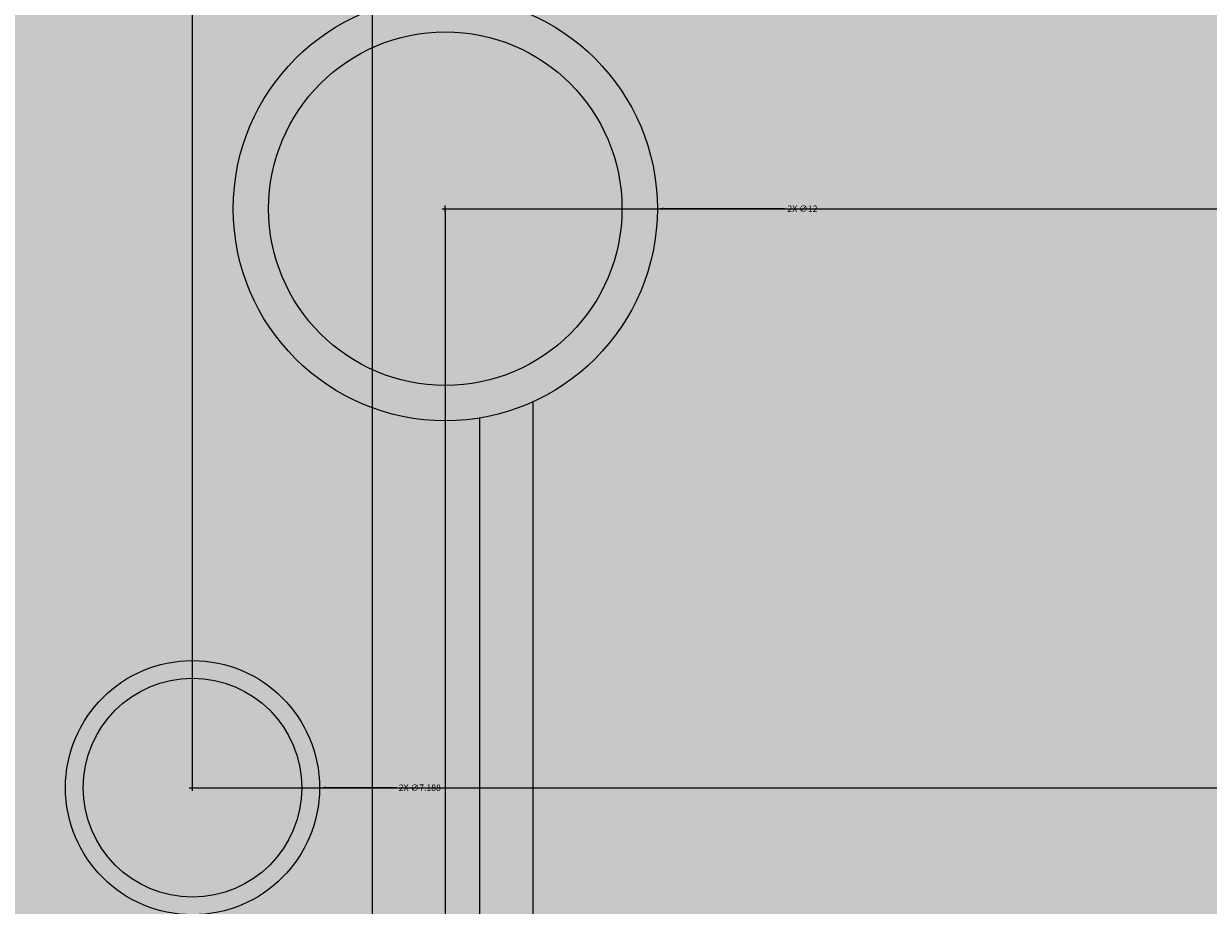
# Model space of a CAD drawing. Units: inches. Extents: x 4508 to 4723, y 847 to 1020.
# Tile 28 of 32: x 4657 to 4691, y 954 to 979. Entities that reach past the tile are written whole.
import ezdxf

# ---------------------------------------------------------------- set-up
doc = ezdxf.new("R2010")
doc.units = ezdxf.units.IN
for name, color, linetype, lineweight in [('A-ANNO-DIMS', 2, 'Continuous', 18), ('A-WALL-DECO', 6, 'Continuous', 18), ('A-WALL-PATT', 254, 'Continuous', 13)]:
    doc.layers.add(name, color=color, linetype=linetype, lineweight=lineweight)
doc.styles.get("Standard").update_dxf_attribs({"font": 'arial.ttf'})
doc.dimstyles.get("Standard").update_dxf_attribs({"dimtxt": 0.18, "dimasz": 0.18, "dimexe": 0.18, "dimexo": 0.0625, "dimgap": 0.09, "dimtad": 0, "dimtih": 1, "dimtoh": 1, "dimdec": 4, "dimzin": 0, "dimdsep": 46, "dimtxsty": 'Standard', "dimcen": 0.09, "dimadec": 0, "dimazin": 0, "dimtfac": 1, "dimtdec": 4, "dimtofl": 0, "dimtmove": 0, "dimatfit": 3, "dimfxl": 1, "dimtolj": 1, "dimtzin": 0, "dimarcsym": 0})

# ---------------------------------------------------------------- blocks, each defined once
blk = doc.blocks.new('*D7')
at = {"layer": 'A-ANNO-DIMS', "color": 0, "lineweight": -2, "transparency": 16777216}
for p, q in [((4588.994, 994.809), (4588.994, 1002.877)), ((4589.174, 1002.697), (4625.189, 1002.697)), ((4661.991, 1002.697), (4625.975, 1002.697)), ((4662.171, 957.665), (4662.171, 1002.877))]:
    blk.add_line(p, q, dxfattribs=at)
at = {"layer": 'A-ANNO-DIMS', "color": 0, "lineweight": 9, "transparency": 16777216}
for points in [[(4589.174, 1002.727), (4589.174, 1002.667), (4588.994, 1002.697)], [(4661.991, 1002.727), (4661.991, 1002.667), (4662.171, 1002.697)]]:
    blk.add_solid(points, dxfattribs=at)
at = {"layer": 'Defpoints', "color": 0, "lineweight": 9, "transparency": 16777216}
for p in [(4662.171, 1002.697), (4588.994, 994.747), (4662.171, 957.602)]:
    blk.add_point(p, dxfattribs=at)
at = {"layer": 'A-ANNO-DIMS', "color": 0, "transparency": 16777216, "insert": (4625.582, 1002.697), "char_height": 0.18, "attachment_point": 5}
blk.add_mtext('\\A1;73.18', dxfattribs=at)
blk = doc.blocks.new('*D8')
at = {"layer": 'A-ANNO-DIMS', "color": 0, "lineweight": -2, "transparency": 16777216}
for p, q in [((4662.171, 957.665), (4662.171, 1002.877)), ((4662.351, 1002.697), (4664.34, 1002.697)), ((4667.082, 1002.697), (4665.092, 1002.697)), ((4667.262, 936.184), (4667.262, 1002.877))]:
    blk.add_line(p, q, dxfattribs=at)
at = {"layer": 'A-ANNO-DIMS', "color": 0, "lineweight": 9, "transparency": 16777216}
for points in [[(4662.351, 1002.727), (4662.351, 1002.667), (4662.171, 1002.697)], [(4667.082, 1002.727), (4667.082, 1002.667), (4667.262, 1002.697)]]:
    blk.add_solid(points, dxfattribs=at)
at = {"layer": 'Defpoints', "color": 0, "lineweight": 9, "transparency": 16777216}
for p in [(4667.262, 1002.697), (4662.171, 957.602), (4667.262, 936.122)]:
    blk.add_point(p, dxfattribs=at)
at = {"layer": 'A-ANNO-DIMS', "color": 0, "transparency": 16777216, "insert": (4664.716, 1002.697), "char_height": 0.18, "attachment_point": 5}
blk.add_mtext('\\A1;5.091', dxfattribs=at)
blk = doc.blocks.new('*D9')
at = {"layer": 'A-ANNO-DIMS', "color": 0, "lineweight": -2, "transparency": 16777216}
for p, q in [((4667.262, 936.184), (4667.262, 1002.877)), ((4667.442, 1002.697), (4668.461, 1002.697)), ((4670.126, 1002.697), (4669.107, 1002.697)), ((4670.306, 994.809), (4670.306, 1002.877))]:
    blk.add_line(p, q, dxfattribs=at)
at = {"layer": 'A-ANNO-DIMS', "color": 0, "lineweight": 9, "transparency": 16777216}
for points in [[(4667.442, 1002.727), (4667.442, 1002.667), (4667.262, 1002.697)], [(4670.126, 1002.727), (4670.126, 1002.667), (4670.306, 1002.697)]]:
    blk.add_solid(points, dxfattribs=at)
at = {"layer": 'Defpoints', "color": 0, "lineweight": 9, "transparency": 16777216}
for p in [(4670.306, 1002.697), (4670.306, 994.747), (4667.262, 936.122)]:
    blk.add_point(p, dxfattribs=at)
at = {"layer": 'A-ANNO-DIMS', "color": 0, "transparency": 16777216, "insert": (4668.784, 1002.697), "char_height": 0.18, "attachment_point": 5}
blk.add_mtext('\\A1;3.04', dxfattribs=at)
blk = doc.blocks.new('*D13')
at = {"layer": 'A-ANNO-DIMS', "color": 0, "lineweight": -2, "transparency": 16777216}
for p, q in [((4669.325, 973.916), (4669.325, 866.617)), ((4689.994, 874.684), (4689.994, 866.617)), ((4669.505, 866.797), (4679.264, 866.797)), ((4689.814, 866.797), (4680.054, 866.797))]:
    blk.add_line(p, q, dxfattribs=at)
at = {"layer": 'A-ANNO-DIMS', "color": 0, "lineweight": 9, "transparency": 16777216}
for points in [[(4669.505, 866.827), (4669.505, 866.767), (4669.325, 866.797)], [(4689.814, 866.827), (4689.814, 866.767), (4689.994, 866.797)]]:
    blk.add_solid(points, dxfattribs=at)
at = {"layer": 'Defpoints', "color": 0, "lineweight": 9, "transparency": 16777216}
for p in [(4669.325, 973.978), (4689.994, 874.747), (4689.994, 866.797)]:
    blk.add_point(p, dxfattribs=at)
at = {"layer": 'A-ANNO-DIMS', "color": 0, "transparency": 16777216, "insert": (4679.659, 866.797), "char_height": 0.18, "attachment_point": 5}
blk.add_mtext('\\A1;20.67', dxfattribs=at)
blk = doc.blocks.new('*D21')
at = {"layer": 'A-ANNO-DIMS', "color": 0, "lineweight": -2, "transparency": 16777216}
for p, q in [((4662.233, 957.602), (4702.124, 957.602)), ((4701.944, 957.422), (4701.944, 947.044)), ((4701.944, 936.302), (4701.944, 946.68)), ((4667.324, 936.122), (4702.124, 936.122))]:
    blk.add_line(p, q, dxfattribs=at)
at = {"layer": 'A-ANNO-DIMS', "color": 0, "lineweight": 9, "transparency": 16777216}
for points in [[(4701.914, 957.422), (4701.974, 957.422), (4701.944, 957.602)], [(4701.914, 936.302), (4701.974, 936.302), (4701.944, 936.122)]]:
    blk.add_solid(points, dxfattribs=at)
at = {"layer": 'Defpoints', "color": 0, "lineweight": 9, "transparency": 16777216}
for p in [(4662.171, 957.602), (4701.944, 957.602), (4667.262, 936.122)]:
    blk.add_point(p, dxfattribs=at)
at = {"layer": 'A-ANNO-DIMS', "color": 0, "transparency": 16777216, "insert": (4701.944, 946.862), "char_height": 0.18, "attachment_point": 5}
blk.add_mtext('\\A1;21.48', dxfattribs=at)
blk = doc.blocks.new('*D22')
at = {"layer": 'A-ANNO-DIMS', "color": 0, "lineweight": -2, "transparency": 16777216}
for p, q in [((4669.387, 973.978), (4702.124, 973.978)), ((4701.944, 973.798), (4701.944, 965.972)), ((4701.944, 957.782), (4701.944, 965.608)), ((4662.233, 957.602), (4702.124, 957.602))]:
    blk.add_line(p, q, dxfattribs=at)
at = {"layer": 'A-ANNO-DIMS', "color": 0, "lineweight": 9, "transparency": 16777216}
for points in [[(4701.914, 973.798), (4701.974, 973.798), (4701.944, 973.978)], [(4701.914, 957.782), (4701.974, 957.782), (4701.944, 957.602)]]:
    blk.add_solid(points, dxfattribs=at)
at = {"layer": 'Defpoints', "color": 0, "lineweight": 9, "transparency": 16777216}
for p in [(4669.325, 973.978), (4701.944, 973.978), (4662.171, 957.602)]:
    blk.add_point(p, dxfattribs=at)
at = {"layer": 'A-ANNO-DIMS', "color": 0, "transparency": 16777216, "insert": (4701.944, 965.79), "char_height": 0.18, "attachment_point": 5}
blk.add_mtext('\\A1;16.376', dxfattribs=at)
blk = doc.blocks.new('*D23')
at = {"layer": 'A-ANNO-DIMS', "color": 0, "lineweight": -2, "transparency": 16777216}
for p, q in [((4694.056, 994.747), (4702.124, 994.747)), ((4701.944, 994.567), (4701.944, 984.545)), ((4701.944, 974.158), (4701.944, 984.181)), ((4669.387, 973.978), (4702.124, 973.978))]:
    blk.add_line(p, q, dxfattribs=at)
at = {"layer": 'A-ANNO-DIMS', "color": 0, "lineweight": 9, "transparency": 16777216}
for points in [[(4701.914, 994.567), (4701.974, 994.567), (4701.944, 994.747)], [(4701.914, 974.158), (4701.974, 974.158), (4701.944, 973.978)]]:
    blk.add_solid(points, dxfattribs=at)
at = {"layer": 'Defpoints', "color": 0, "lineweight": 9, "transparency": 16777216}
for p in [(4693.994, 994.747), (4701.944, 994.747), (4669.325, 973.978)]:
    blk.add_point(p, dxfattribs=at)
at = {"layer": 'A-ANNO-DIMS', "color": 0, "transparency": 16777216, "insert": (4701.944, 984.363), "char_height": 0.18, "attachment_point": 5}
blk.add_mtext('\\A1;20.77', dxfattribs=at)
blk = doc.blocks.new('*D44')
at = {"layer": 'A-ANNO-DIMS', "color": 0, "lineweight": -2, "transparency": 16777216}
for p, q in [((4669.235, 973.978), (4669.415, 973.978)), ((4669.325, 973.888), (4669.325, 974.068)), ((4678.925, 973.978), (4675.505, 973.978))]:
    blk.add_line(p, q, dxfattribs=at)
at = {"layer": 'A-ANNO-DIMS', "color": 0, "lineweight": 9, "transparency": 16777216}
blk.add_solid([(4675.505, 974.008), (4675.505, 973.948), (4675.325, 973.978)], dxfattribs=at)
at = {"layer": 'Defpoints', "color": 0, "lineweight": 9, "transparency": 16777216}
for p in [(4663.325, 973.979), (4675.325, 973.978)]:
    blk.add_point(p, dxfattribs=at)
at = {"layer": 'A-ANNO-DIMS', "color": 0, "transparency": 16777216, "insert": (4679.431, 973.978), "char_height": 0.18, "attachment_point": 5}
blk.add_mtext('\\A1;2X ∅12', dxfattribs=at)
blk = doc.blocks.new('*D46')
at = {"layer": 'A-ANNO-DIMS', "color": 0, "lineweight": -2, "transparency": 16777216}
for p, q in [((4662.081, 957.602), (4662.261, 957.602)), ((4662.171, 957.512), (4662.171, 957.692)), ((4667.921, 957.602), (4665.945, 957.602))]:
    blk.add_line(p, q, dxfattribs=at)
at = {"layer": 'A-ANNO-DIMS', "color": 0, "lineweight": 9, "transparency": 16777216}
blk.add_solid([(4665.945, 957.632), (4665.945, 957.572), (4665.765, 957.602)], dxfattribs=at)
at = {"layer": 'Defpoints', "color": 0, "lineweight": 9, "transparency": 16777216}
for p in [(4658.576, 957.602), (4665.765, 957.602)]:
    blk.add_point(p, dxfattribs=at)
at = {"layer": 'A-ANNO-DIMS', "color": 0, "transparency": 16777216, "insert": (4668.603, 957.602), "char_height": 0.18, "attachment_point": 5}
blk.add_mtext('\\A1;2X ∅7.188', dxfattribs=at)

msp = doc.modelspace()

# ---------------------------------------------------------------- hatches: boundary and pattern name
at = {"layer": 'A-WALL-PATT', "transparency": 33554508}
h = msp.add_hatch(color=256, dxfattribs=at)
h.dxf.hatch_style = 1
h.paths.add_polyline_path([(4661.6706, 954.043, -0.3739004), (4658.5765, 957.6021, -1), (4665.7646, 957.6021, -0.3739004), (4662.6706, 954.043), (4662.6706, 944.4021, -0.2114781), (4670.3062, 945.0869), (4670.3062, 968.0592, -0.4632086), (4663.3246, 973.9783, -0.4632086), (4670.3062, 979.8975), (4670.3062, 994.7469), (4588.9938, 994.7469), (4588.9938, 904.7469), (4657.9938, 904.7469), (4657.9938, 886.7469), (4549.9938, 886.7469), (4549.9938, 878.7469), (4693.9938, 878.7469), (4693.9938, 994.7469), (4671.8062, 994.7469), (4671.8062, 979.4411, -0.2941682), (4675.3246, 973.9783, -0.2941682), (4671.8062, 968.5156), (4671.8062, 944.4278, -0.2741114), (4676.7298, 936.1217, -0.2741114), (4671.8062, 927.8155), (4671.8062, 907.6998, -0.3779645), (4677.0562, 901.7469, -0.3779645), (4671.8062, 895.7939), (4671.8062, 883.7469), (4670.3062, 883.7469), (4670.3062, 895.7939, -0.3779645), (4665.0562, 901.7469, -0.3779645), (4670.3062, 907.6998), (4670.3062, 927.1564, -0.2114781), (4662.6706, 927.8412), (4662.6706, 918.2003, -0.3739004), (4665.7646, 914.6412, -1), (4658.5765, 914.6412, -0.3739004), (4661.6706, 918.2003), (4661.6706, 928.4807, -0.2391825), (4657.7936, 936.1217, -0.2391825), (4661.6706, 943.7626)])
at = {"layer": 'A-WALL-PATT', "transparency": 33554681}
h = msp.add_hatch(color=256, dxfattribs=at)
h.dxf.hatch_style = 1
h.paths.add_polyline_path([(4671.8062, 968.5156, -0.0656104), (4670.3062, 968.0592), (4670.3062, 945.0869, -0.0433429), (4671.8062, 944.4278)])
h.paths.add_polyline_path([(4662.6706, 954.043, -0.0698991), (4661.6706, 954.043), (4661.6706, 943.7626, -0.0313734), (4662.6706, 944.4021)])
h.paths.add_polyline_path([(4665.7646, 957.6021, 1), (4658.5765, 957.6021, 1)])
h.paths.add_polyline_path([(4659.0765, 957.6021, -1), (4665.2646, 957.6021, -1)], flags=16)
h.paths.add_polyline_path([(4675.3246, 973.9783, 1), (4663.3246, 973.9783, 1)])
h.paths.add_polyline_path([(4664.3246, 973.9783, -1), (4674.3246, 973.9783, -1)], flags=16)
h.paths.add_polyline_path([(4671.8062, 994.7469), (4670.3062, 994.7469), (4670.3062, 979.8975, -0.0656104), (4671.8062, 979.4411)])
at = {"layer": 'A-WALL-PATT', "transparency": 33554556}
h = msp.add_hatch(color=256, dxfattribs=at)
h.dxf.hatch_style = 1
h.paths.add_polyline_path([(4676.0562, 901.7469, 1), (4666.0562, 901.7469, 1)])
h.paths.add_polyline_path([(4659.0765, 914.6412, 1), (4665.2646, 914.6412, 1)])
h.paths.add_polyline_path([(4675.7298, 936.1217, 1), (4658.7936, 936.1217, 1)])
h.paths.add_polyline_path([(4659.0765, 957.6021, 1), (4665.2646, 957.6021, 1)])
h.paths.add_polyline_path([(4664.3246, 973.9783, 1), (4674.3246, 973.9783, 1)])

# ---------------------------------------------------------------- linework, layer by layer
at = {"layer": 'A-WALL-DECO'}
for p, q in [((4671.8062, 944.4278), (4671.8062, 968.5156)), ((4670.3062, 945.0869), (4670.3062, 968.0592))]:
    msp.add_line(p, q, dxfattribs=at)
for centre, radius in [((4669.3246, 973.9783), 6), ((4669.3246, 973.9783), 5), ((4662.1706, 957.6021), 3.5941), ((4662.1706, 957.6021), 3.0941)]:
    msp.add_circle(centre, radius, dxfattribs=at)

# ---------------------------------------------------------------- dimensions: what is measured, and where the dimension line sits
at = {"layer": 'A-ANNO-DIMS'}
for base, p1, p2, override, picture, middle in [((4662.1706, 1002.6969), (4588.9938, 994.7469), (4662.1706, 957.6021), {"dimdec": 2, "dimlfac": 1, "dimrnd": 0, "dimzin": 0, "dimdsep": 46, "dimlunit": 2}, '*D7', (4625.5822, 1002.6969)), ((4667.2617, 1002.6969), (4662.1706, 957.6021), (4667.2617, 936.1217), {"dimdec": 3, "dimlfac": 1, "dimrnd": 0, "dimzin": 0, "dimdsep": 46, "dimlunit": 2}, '*D8', (4664.7161, 1002.6969)), ((4670.3062, 1002.6969), (4667.2617, 936.1217), (4670.3062, 994.7469), {"dimdec": 2, "dimlfac": 1, "dimrnd": 0, "dimzin": 0, "dimdsep": 46, "dimlunit": 2}, '*D9', (4668.7839, 1002.6969)), ((4689.9938, 866.7969), (4669.3246, 973.9783), (4689.9938, 874.7469), {"dimdec": 2, "dimlfac": 1, "dimrnd": 0, "dimzin": 0, "dimdsep": 46, "dimlunit": 2}, '*D13', (4679.6592, 866.7969))]:
    dim = msp.add_linear_dim(base=base, p1=p1, p2=p2, dimstyle='Standard', override=override, dxfattribs=at)
    dim.commit()
    dim.dimension.update_dxf_attribs({"geometry": picture, "text_midpoint": middle})
for base, p1, p2, override, picture, middle in [((4701.9438, 994.7469), (4669.3246, 973.9783), (4693.9938, 994.7469), {"dimdec": 2, "dimlfac": 1, "dimrnd": 0, "dimzin": 0, "dimdsep": 46, "dimlunit": 2}, '*D23', (4701.9438, 984.3626)), ((4701.9438, 973.9783), (4662.1706, 957.6021), (4669.3246, 973.9783), {"dimdec": 3, "dimlfac": 1, "dimrnd": 0, "dimzin": 0, "dimdsep": 46, "dimlunit": 2}, '*D22', (4701.9438, 965.7902)), ((4701.9438, 957.6021), (4667.2617, 936.1217), (4662.1706, 957.6021), {"dimdec": 2, "dimlfac": 1, "dimrnd": 0, "dimzin": 0, "dimdsep": 46, "dimlunit": 2}, '*D21', (4701.9438, 946.8619))]:
    dim = msp.add_linear_dim(base=base, p1=p1, p2=p2, angle=90, dimstyle='Standard', override=override, dxfattribs=at)
    dim.commit()
    dim.dimension.update_dxf_attribs({"geometry": picture, "text_midpoint": middle})
for p1, p2, override, picture, middle in [((4663.3246, 973.9787), (4675.3246, 973.978), {"dimdec": 0, "dimlfac": 1, "dimrnd": 0, "dimzin": 0, "dimdsep": 46, "dimlunit": 2}, '*D44', (4678.9246, 973.9778)), ((4658.5765, 957.6022), (4665.7646, 957.602), {"dimdec": 3, "dimlfac": 1, "dimrnd": 0, "dimzin": 0, "dimdsep": 46, "dimlunit": 2}, '*D46', (4667.9211, 957.6019))]:
    dim = msp.add_diameter_dim_2p(p1=p1, p2=p2, text='2X <>', dimstyle='Standard', override=override, dxfattribs=at)
    dim.commit()
    dim.dimension.update_dxf_attribs({"geometry": picture, "text_midpoint": middle, "dimtype": 163})

doc.saveas('drawing.dxf')
